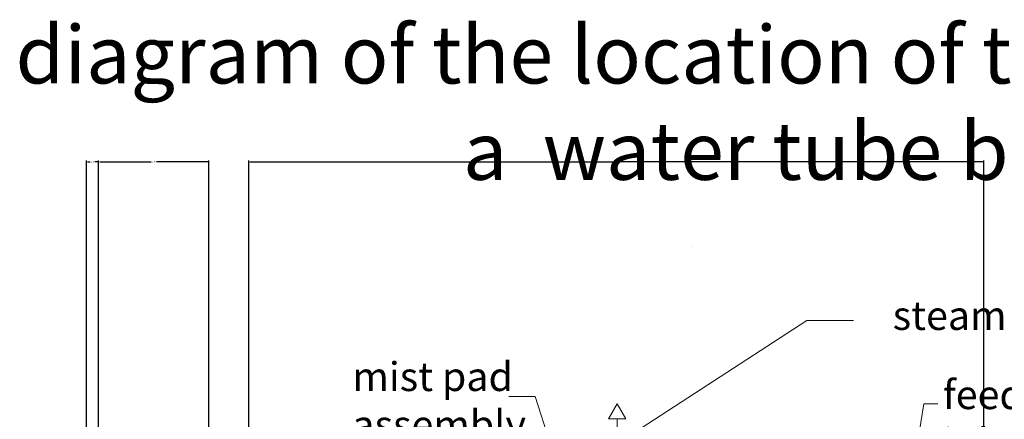
# Model space of a CAD drawing. Units: inches. Extents: x -1 to 292, y -3 to 199.
# Tile 32 of 52: x 10 to 181, y 130 to 199. Entities that reach past the tile are written whole.
import ezdxf

# ---------------------------------------------------------------- set-up
doc = ezdxf.new("R2010")
doc.units = ezdxf.units.IN
doc.header["$MEASUREMENT"] = 0
for name, color, linetype, lineweight in [('M-ANNO-LEAD', 2, 'Continuous', 18), ('M-ANNO-SYMB', 1, 'Continuous', 18), ('M-ANNO-TEXT', 3, 'Continuous', 25), ('M-DIMS', 2, 'Continuous', 18), ('M-EQPM', 7, 'Continuous', 35)]:
    doc.layers.add(name, color=color, linetype=linetype, lineweight=lineweight)
doc.styles.get("Standard").update_dxf_attribs({"font": 'arial.ttf'})
doc.dimstyles.get("Standard").update_dxf_attribs({"dimtxt": 0.18, "dimasz": 0.18, "dimexe": 0.18, "dimexo": 0.0625, "dimgap": 0.09, "dimtad": 0, "dimtih": 1, "dimtoh": 1, "dimdec": 4, "dimzin": 0, "dimdsep": 46, "dimtxsty": 'Standard', "dimcen": 0.09, "dimadec": 0, "dimazin": 0, "dimtfac": 1, "dimtdec": 4, "dimtofl": 0, "dimtmove": 0, "dimatfit": 3, "dimfxl": 1, "dimtolj": 1, "dimtzin": 0, "dimarcsym": 0})

# ---------------------------------------------------------------- blocks, each defined once
blk = doc.blocks.new('ARROW-STEAM-OUT')
blk.add_line((113.61, 129.86), (113.61, 124.67))
blk.add_lwpolyline([(112.11, 129.86), (115.11, 129.86), (113.61, 132.46)], close=True)
blk = doc.blocks.new('*D9')
at = {"layer": 'Defpoints', "color": 0, "transparency": 16777216}
for p in [(177.05, 174.36), (49.92, 99.77), (177.05, 99.77)]:
    blk.add_point(p, dxfattribs=at)
at = {"layer": 'M-DIMS', "color": 0, "lineweight": -2, "transparency": 16777216}
for p, q in [((49.92, 99.84), (49.92, 174.54)), ((50.1, 174.36), (113.03, 174.36)), ((176.87, 174.36), (113.94, 174.36)), ((177.05, 99.84), (177.05, 174.54))]:
    blk.add_line(p, q, dxfattribs=at)
at = {"layer": 'M-DIMS', "color": 0, "transparency": 16777216}
for points in [[(50.1, 174.39), (50.1, 174.33), (49.92, 174.36)], [(176.87, 174.39), (176.87, 174.33), (177.05, 174.36)]]:
    blk.add_solid(points, dxfattribs=at)
at = {"layer": 'M-DIMS', "color": 0, "transparency": 16777216, "insert": (113.49, 174.36), "char_height": 0.18, "attachment_point": 5}
blk.add_mtext('\\A1;127.13', dxfattribs=at)
blk = doc.blocks.new('*D15')
at = {"layer": 'Defpoints', "color": 0, "transparency": 16777216}
for p in [(23.95, 174.36), (21.86, 88.58), (23.95, 88.58)]:
    blk.add_point(p, dxfattribs=at)
at = {"layer": 'M-DIMS', "color": 0, "lineweight": -2, "transparency": 16777216}
for p, q in [((21.86, 88.64), (21.86, 174.54)), ((22.04, 174.36), (22.51, 174.36)), ((23.77, 174.36), (23.3, 174.36)), ((23.95, 88.64), (23.95, 174.54))]:
    blk.add_line(p, q, dxfattribs=at)
at = {"layer": 'M-DIMS', "color": 0, "transparency": 16777216}
for points in [[(22.04, 174.39), (22.04, 174.33), (21.86, 174.36)], [(23.77, 174.39), (23.77, 174.33), (23.95, 174.36)]]:
    blk.add_solid(points, dxfattribs=at)
at = {"layer": 'M-DIMS', "color": 0, "transparency": 16777216, "insert": (22.91, 174.36), "char_height": 0.18, "attachment_point": 5}
blk.add_mtext('\\A1;2.089', dxfattribs=at)
blk = doc.blocks.new('*D16')
at = {"layer": 'Defpoints', "color": 0, "transparency": 16777216}
for p in [(43, 174.36), (43, 93.64), (23.95, 85.56)]:
    blk.add_point(p, dxfattribs=at)
at = {"layer": 'M-DIMS', "color": 0, "lineweight": -2, "transparency": 16777216}
for p, q in [((23.95, 85.62), (23.95, 174.54)), ((24.13, 174.36), (33.02, 174.36)), ((42.82, 174.36), (33.93, 174.36)), ((43, 93.7), (43, 174.54))]:
    blk.add_line(p, q, dxfattribs=at)
at = {"layer": 'M-DIMS', "color": 0, "transparency": 16777216}
for points in [[(24.13, 174.39), (24.13, 174.33), (23.95, 174.36)], [(42.82, 174.39), (42.82, 174.33), (43, 174.36)]]:
    blk.add_solid(points, dxfattribs=at)
at = {"layer": 'M-DIMS', "color": 0, "transparency": 16777216, "insert": (33.47, 174.36), "char_height": 0.18, "attachment_point": 5}
blk.add_mtext('\\A1;19.047', dxfattribs=at)

msp = doc.modelspace()

# ---------------------------------------------------------------- linework, layer by layer
at = {"layer": 'M-ANNO-LEAD'}
for p, q in [((115.4883, 126.765), (146.4422, 146.8667)), ((146.4422, 146.8667), (154.5322, 146.8667)), ((99.4422, 133.7141), (94.876, 133.7141)), ((108.0603, 106.9941), (99.4422, 133.7141)), ((162.951, 109.7655), (166.6813, 132.451)), ((166.6813, 132.451), (169.106, 132.451))]:
    msp.add_line(p, q, dxfattribs=at)
at = {"layer": 'M-EQPM'}
msp.add_lwpolyline([(126.6686, 159.7627), (126.6686, 159.7627)], close=True, dxfattribs=at)

# ---------------------------------------------------------------- block references
at = {"layer": 'M-ANNO-SYMB'}
msp.add_blockref('ARROW-STEAM-OUT', (0, 0), dxfattribs=at)

# ---------------------------------------------------------------- texts
at = {"layer": 'M-ANNO-TEXT', "attachment_point": 1}
for s, width, heights, insert, char_height in [('\\pxqc;diagram of the location of the mud drum on a  water tube boiler', 286.43424, [43.6883], (5.3019, 197.8921), 10), ('steam outlet', 40.442607, [0], (161.2863, 150.2478), 5), ('mist pad \\Passembly', 40.442607, [0], (67.8309, 139.6846), 5), ('feed water inlet', 47.899539, [0], (169.9729, 136.5612), 5)]:
    msp.add_mtext_dynamic_manual_height_columns(s, width=width, gutter_width=1, heights=heights, dxfattribs=dict(at, insert=insert, char_height=char_height))

# ---------------------------------------------------------------- dimensions: what is measured, and where the dimension line sits
at = {"layer": 'M-DIMS'}
for base, p1, p2, override, picture, middle in [((23.9502, 174.3627), (21.8612, 88.5821), (23.9502, 88.5821), {"dimdec": 3, "dimlfac": 1, "dimrnd": 0, "dimzin": 0, "dimdsep": 46, "dimlunit": 2}, '*D15', (22.9057, 174.3627)), ((42.99769, 174.3627), (23.95023, 85.55517), (42.99769, 93.64034), {"dimdec": 3, "dimlfac": 1, "dimrnd": 0, "dimzin": 0, "dimdsep": 46, "dimlunit": 2}, '*D16', (33.47396, 174.3627)), ((177.0526, 174.3627), (49.9241, 99.7735), (177.0526, 99.7735), {"dimdec": 2, "dimlfac": 1, "dimrnd": 0, "dimzin": 0, "dimdsep": 46, "dimlunit": 2}, '*D9', (113.4883, 174.3627))]:
    dim = msp.add_linear_dim(base=base, p1=p1, p2=p2, dimstyle='Standard', override=override, dxfattribs=at)
    dim.commit()
    dim.dimension.update_dxf_attribs({"geometry": picture, "text_midpoint": middle})

doc.saveas('drawing.dxf')
